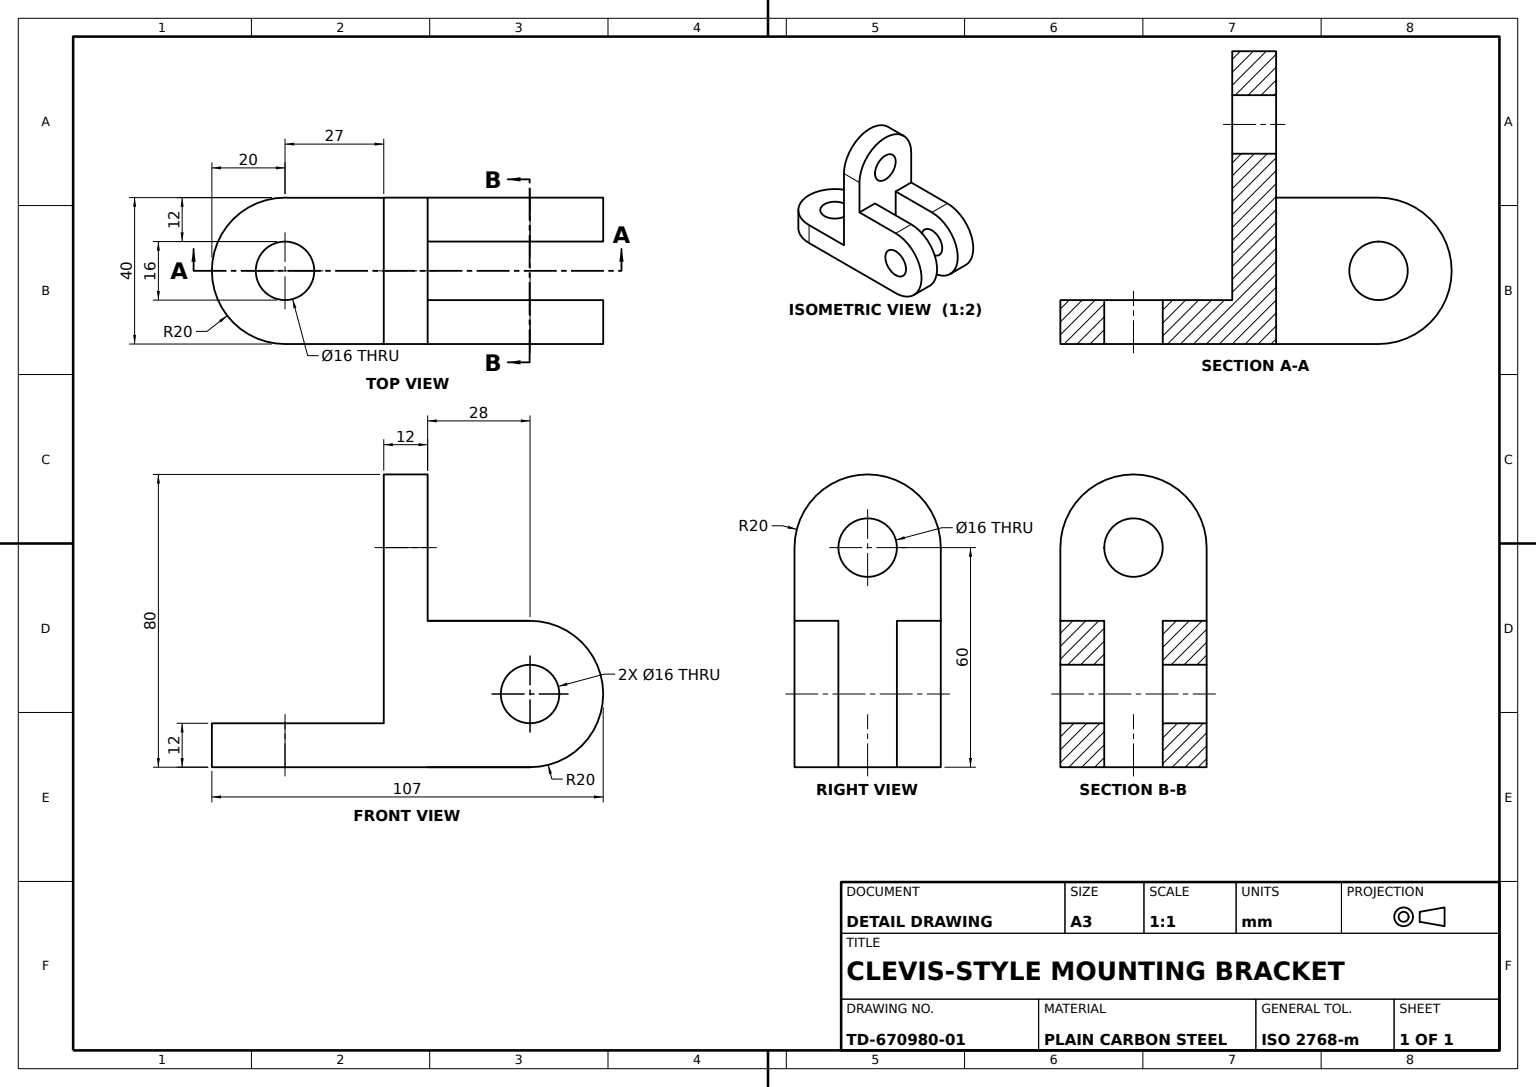
SolidWorks part; units mm, degrees
material "Plain Carbon Steel"
ref_plane "Front Plane" through (0, 0, 0) normal (0, 0, 1) x (1, 0, 0)
ref_plane "Top Plane" through (0, 0, 0) normal (0, 1, 0) x (1, 0, 0)
ref_plane "Right Plane" through (0, 0, 0) normal (1, 0, 0) x (0, 0, -1)
sketch "Upright Lug Sketch" plane through (0, 0, 0) normal (0, 0, 1) x (1, 0, 0)
  line L0 (0, 73.8028) -> (0, -88.4507) construction
  line L1 (-122.1408, 0) -> (126.8732, 0) construction
  line L3 (-20, 0) -> (20, 0)
  line L4 (-20, 0) -> (-20, 60)
  line L6 (20, 0) -> (20, 60)
  arc A0 (20, 60) -> (-20, 60) centre (0, 60) ccw
  circle A1 centre (0, 60) radius 8
  dimension "D3" = 40
  dimension "D4" = 16
  dimension "D1" = 60
  dimension "D2" = 40
extrude "Upright Lug" add sketch "Upright Lug Sketch" along normal blind 12
sketch "Clevis Side Lug Sketch" plane through (20, 0, 0) normal (1, 0, 0) x (0, 0, -1)
  line L1 (0, 0) -> (-40, 0)
  line L2 (0, 0) -> (0, 40)
  line L3 (0, 40) -> (-40, 40)
  arc A0 (-40, 40) -> (-40, 0) centre (-40, 20) ccw
  circle A1 centre (-40, 20) radius 8
  dimension "D3" = 40
  dimension "D4" = 16
  dimension "D1" = 40
  dimension "D2" = 40
extrude "Clevis Side Lug" add sketch "Clevis Side Lug Sketch" against normal blind 12
mirror "Clevis Side Lug Mirror" about plane through (0, 0, 0) normal (1, 0, 0) of "Clevis Side Lug"
sketch "Horizontal Lug Sketch" plane through (0, 0, 0) normal (0, -1, 0) x (1, 0, 0)
  line L0 (-28.8554, 0) -> (39.8502, 0) construction
  line L1 (-20, 40) -> (-20, 0) construction
  line L2 (-20, 12) -> (19.9618, 12)
  line L3 (-20, 12) -> (-20, -27)
  line L5 (19.9618, 12) -> (19.9618, -25.7637)
  line L7 (8, 40) -> (20, 40) construction
  arc A0 (-20, -27) -> (19.9618, -25.7637) centre (0, -27) ccw
  circle A1 centre (0, -27) radius 8
  dimension "D3" = 40
  dimension "D4" = 16
  dimension "D1" = 12
  dimension "D2" = 65.7637
  dimension "40" = 39.9618
extrude "Horizontal Lug" add sketch "Horizontal Lug Sketch" against normal blind 12
